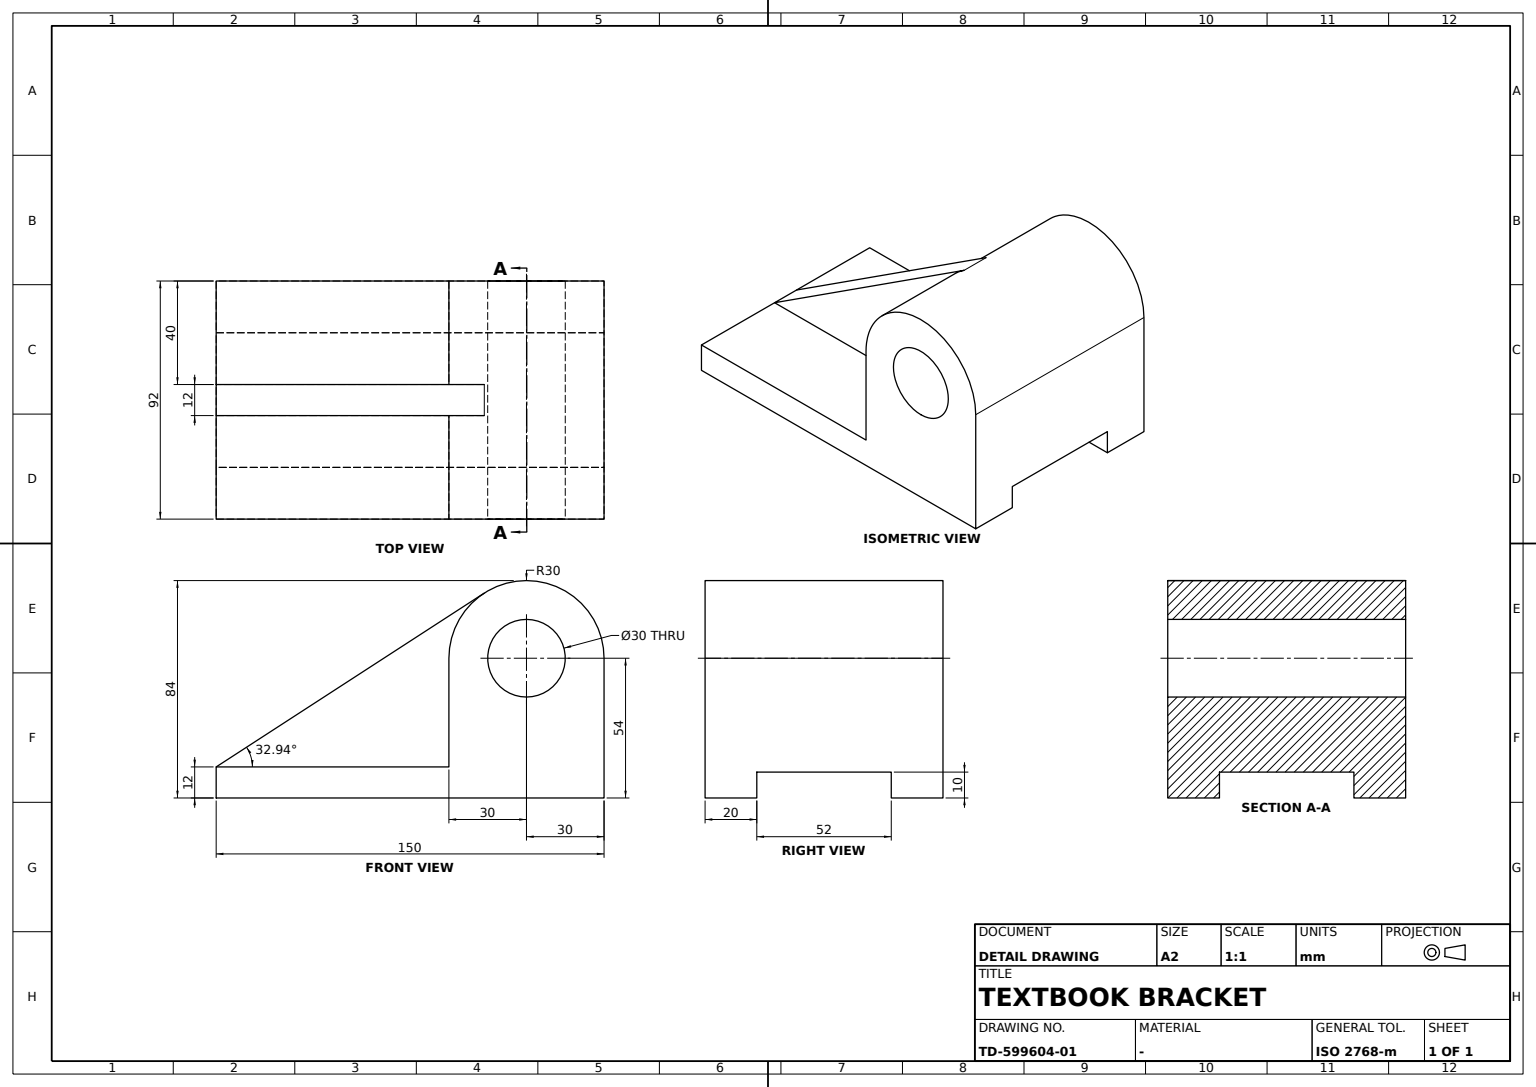
CATIA V5 part; units mm, degrees
sketch "Sketch1" plane through (0, 0, 0) normal (1, 0, 0) x (0, 1, 0)
  line L0 (0, 0) -> (150, 0)
  line L1 (150, 0) -> (150, 54)
  arc A0 (150, 54) -> (90, 54) centre (120, 54) ccw
  point P0 (120, 54)
  line L2 (90, 54) -> (90, 12)
  line L3 (90, 12) -> (0, 12)
  point P1 (0, 12)
  line L4 (0, 12) -> (0, 0)
  circle A1 centre (120, 54) radius 15
  dimension "length L4" = 12
  dimension "radius A0" = 30
  dimension "length L2" = 42
  dimension "distance L1 y axis" = 150
  dimension "radius A1" = 15
  dimension "distance P0 L0" = 54
  constraint horizontal L0 x-axis
  constraint horizontal L3 x-axis
  constraint vertical L1 y-axis
  constraint vertical L2 y-axis
  constraint vertical L4 y-axis
  constraint tangency A0 L1
  constraint coincidence P1 y-axis
extrude "Pad1" add sketch "Sketch1" along normal mid plane 92
sketch "Sketch2" plane through (0, 0, 0) normal (1, 0, 0) x (0, 1, 0)
  line L0 (103.6878, 79.1776) -> (0, 12)
  point P0 (103.6878, 79.1776)
  point P1 (0, 12)
  point P2 (0, 12)
  arc A0 (150, 54) -> (90, 54) centre (120, 54) ccw construction
  constraint coincidence P1 P2
  constraint coincidence P0 A0
  constraint tangency L0 A0
rib "Stiffener1" sketch "Sketch2" thickness 12 sides both
sketch "Sketch3" plane through (0, 150, 0) normal (0, 1, 0) x (-1, 0, 0)
  point P0 (-26, 0)
  line L0 (-26, 0) -> (-26, 10)
  line L1 (-26, 10) -> (26, 10)
  line L2 (26, 10) -> (26, 0)
  point P1 (26, 0)
  line L3 (26, 0) -> (-26, 0)
  dimension "length L2" = 10
  dimension "distance L0 L2" = 52
  constraint coincidence P0 x-axis
  constraint coincidence P1 x-axis
  constraint vertical L0 y-axis
  constraint vertical L2 y-axis
  constraint horizontal L1 x-axis
  constraint symmetry L0 L2 y-axis
extrude "Pocket1" cut sketch "Sketch3" against normal up to next
